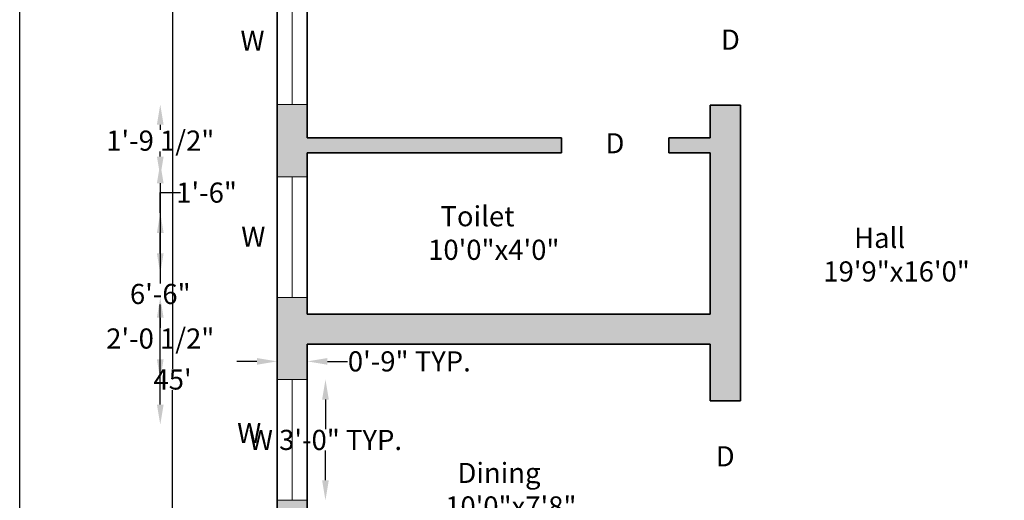
# Model space of a CAD drawing. Units: inches. Extents: x 1054 to 1577, y 4847 to 5610.
# Tile 3 of 5: x 1054 to 1347, y 5221 to 5365. Entities that reach past the tile are written whole.
import ezdxf

# ---------------------------------------------------------------- set-up
doc = ezdxf.new("R2010")
doc.units = ezdxf.units.IN
doc.header["$MEASUREMENT"] = 0
for name, color, linetype, lineweight in [('A-ANNO-DIMS', 2, 'Continuous', 18), ('A-ANNO-TEXT', 7, 'Continuous', 18), ('A-ANNO-TTLB', 7, 'Continuous', 25), ('A-AREA-IDEN', 7, 'Continuous', 18), ('A-GLAZ', 4, 'Continuous', 18), ('A-WALL', 7, 'Continuous', 35)]:
    doc.layers.add(name, color=color, linetype=linetype, lineweight=lineweight)
doc.layers.add('A-WALL-PATT', color=240, linetype='Continuous', lineweight=13, true_color=0xed1f24)
doc.styles.get("Standard").update_dxf_attribs({"font": 'arial.ttf'})
doc.dimstyles.get("Standard").update_dxf_attribs({"dimtxt": 6, "dimasz": 6, "dimexe": 0.18, "dimexo": 0.0625, "dimgap": 0.09, "dimtad": 0, "dimtih": 1, "dimtoh": 1, "dimdec": 1, "dimzin": 0, "dimdsep": 46, "dimlunit": 3, "dimtxsty": 'Standard', "dimcen": 0.09, "dimse1": 1, "dimse2": 1, "dimadec": 0, "dimazin": 0, "dimtfac": 1, "dimtdec": 1, "dimtofl": 0, "dimtmove": 0, "dimatfit": 3, "dimfxl": 1, "dimtolj": 1, "dimtzin": 0, "dimarcsym": 0})

# ---------------------------------------------------------------- blocks, each defined once
blk = doc.blocks.new('*D5')
at = {"layer": 'A-ANNO-DIMS', "color": 0, "lineweight": -2, "transparency": 16777216}
for p, q in [((1099.63, 5521.48), (1099.63, 5260.62)), ((1099.63, 4993.48), (1099.63, 5254.34))]:
    blk.add_line(p, q, dxfattribs=at)
at = {"layer": 'A-ANNO-DIMS', "color": 0, "transparency": 16777216}
for points in [[(1098.63, 5521.48), (1100.63, 5521.48), (1099.63, 5527.48)], [(1098.63, 4993.48), (1100.63, 4993.48), (1099.63, 4987.48)]]:
    blk.add_solid(points, dxfattribs=at)
at = {"layer": 'Defpoints', "color": 0, "transparency": 16777216}
for p in [(1130.77, 5527.48), (1099.63, 4987.48), (1130.77, 4987.48)]:
    blk.add_point(p, dxfattribs=at)
at = {"layer": 'A-ANNO-DIMS', "color": 0, "transparency": 16777216, "insert": (1099.63, 5257.48), "char_height": 6, "attachment_point": 5}
blk.add_mtext("\\A1;45'", dxfattribs=at)
blk = doc.blocks.new('WINDOW-36IN')
for p, q in [((0, 9), (0, 0)), ((36, 9), (0, 9)), ((36, 0), (36, 9)), ((36, 4.5), (0, 4.5)), ((0, 0), (36, 0))]:
    blk.add_line(p, q)
blk = doc.blocks.new('*D10')
at = {"layer": 'A-ANNO-DIMS', "color": 0, "lineweight": -2, "transparency": 16777216}
for p, q in [((1145.17, 5251.48), (1145.17, 5242.64)), ((1145.17, 5227.48), (1145.17, 5236.33))]:
    blk.add_line(p, q, dxfattribs=at)
at = {"layer": 'A-ANNO-DIMS', "color": 0, "transparency": 16777216}
for points in [[(1144.17, 5251.48), (1146.17, 5251.48), (1145.17, 5257.48)], [(1144.17, 5227.48), (1146.17, 5227.48), (1145.17, 5221.48)]]:
    blk.add_solid(points, dxfattribs=at)
at = {"layer": 'Defpoints', "color": 0, "transparency": 16777216}
for p in [(1139.77, 5257.48), (1139.77, 5221.48), (1145.17, 5221.48)]:
    blk.add_point(p, dxfattribs=at)
at = {"layer": 'A-ANNO-DIMS', "color": 0, "transparency": 16777216, "insert": (1145.17, 5239.48), "char_height": 6, "attachment_point": 5}
blk.add_mtext('\\A1;W 3\'-0" TYP.', dxfattribs=at)
blk = doc.blocks.new('*D11')
at = {"layer": 'A-ANNO-DIMS', "color": 0, "lineweight": -2, "transparency": 16777216}
for p, q in [((1124.77, 5262.88), (1118.77, 5262.88)), ((1145.77, 5262.88), (1151.77, 5262.88))]:
    blk.add_line(p, q, dxfattribs=at)
at = {"layer": 'A-ANNO-DIMS', "color": 0, "transparency": 16777216}
for points in [[(1124.77, 5263.88), (1124.77, 5261.88), (1130.77, 5262.88)], [(1145.77, 5263.88), (1145.77, 5261.88), (1139.77, 5262.88)]]:
    blk.add_solid(points, dxfattribs=at)
at = {"layer": 'Defpoints', "color": 0, "transparency": 16777216}
for p in [(1139.77, 5262.88), (1130.77, 5257.48), (1139.77, 5257.48)]:
    blk.add_point(p, dxfattribs=at)
at = {"layer": 'A-ANNO-DIMS', "color": 0, "transparency": 16777216, "insert": (1170.15, 5262.88), "char_height": 6, "attachment_point": 5}
blk.add_mtext('\\A1;0\'-9" TYP.', dxfattribs=at)
blk = doc.blocks.new('*D25')
at = {"layer": 'A-ANNO-DIMS', "color": 0, "lineweight": -2, "transparency": 16777216}
for p, q in [((1348.59, 4855.83), (1352.52, 4855.83)), ((1372.59, 4855.83), (1368.65, 4855.83))]:
    blk.add_line(p, q, dxfattribs=at)
at = {"layer": 'A-ANNO-DIMS', "color": 0, "transparency": 16777216}
for points in [[(1348.59, 4856.83), (1348.59, 4854.83), (1342.59, 4855.83)], [(1372.59, 4856.83), (1372.59, 4854.83), (1378.59, 4855.83)]]:
    blk.add_solid(points, dxfattribs=at)
at = {"layer": 'Defpoints', "color": 0, "transparency": 16777216}
for p in [(1342.59, 5389.48), (1378.59, 5389.48), (1378.59, 4855.83)]:
    blk.add_point(p, dxfattribs=at)
at = {"layer": 'A-ANNO-DIMS', "color": 0, "transparency": 16777216, "insert": (1360.59, 4855.83), "char_height": 6, "attachment_point": 5}
blk.add_mtext('\\A1;3\'-0"', dxfattribs=at)
blk = doc.blocks.new('*D26')
at = {"layer": 'A-ANNO-DIMS', "color": 0, "lineweight": -2, "transparency": 16777216}
for p, q in [((1221.44, 4855.83), (1223.32, 4855.83)), ((1241.44, 4855.83), (1239.56, 4855.83))]:
    blk.add_line(p, q, dxfattribs=at)
at = {"layer": 'A-ANNO-DIMS', "color": 0, "transparency": 16777216}
for points in [[(1221.44, 4856.83), (1221.44, 4854.83), (1215.44, 4855.83)], [(1241.44, 4856.83), (1241.44, 4854.83), (1247.44, 4855.83)]]:
    blk.add_solid(points, dxfattribs=at)
at = {"layer": 'Defpoints', "color": 0, "transparency": 16777216}
for p in [(1215.44, 5324.98), (1247.44, 5324.98), (1247.44, 4855.83)]:
    blk.add_point(p, dxfattribs=at)
at = {"layer": 'A-ANNO-DIMS', "color": 0, "transparency": 16777216, "insert": (1231.44, 4855.83), "char_height": 6, "attachment_point": 5}
blk.add_mtext('\\A1;2\'-8"', dxfattribs=at)
blk = doc.blocks.new('*D33')
at = {"layer": 'A-ANNO-DIMS', "color": 0, "lineweight": -2, "transparency": 16777216}
for p, q in [((1095.97, 5275.9), (1095.97, 5272.88)), ((1095.97, 5263.48), (1095.97, 5266.5))]:
    blk.add_line(p, q, dxfattribs=at)
at = {"layer": 'A-ANNO-DIMS', "color": 0, "transparency": 16777216}
for points in [[(1094.97, 5275.9), (1096.97, 5275.9), (1095.97, 5281.9)], [(1094.97, 5263.48), (1096.97, 5263.48), (1095.97, 5257.48)]]:
    blk.add_solid(points, dxfattribs=at)
at = {"layer": 'Defpoints', "color": 0, "transparency": 16777216}
for p in [(1095.97, 5281.9), (1130.77, 5281.9), (1130.77, 5257.48)]:
    blk.add_point(p, dxfattribs=at)
at = {"layer": 'A-ANNO-DIMS', "color": 0, "transparency": 16777216, "insert": (1095.97, 5269.69), "char_height": 6, "attachment_point": 5}
blk.add_mtext('\\A1;2\'-0 1/2"', dxfattribs=at)
blk = doc.blocks.new('*D34')
at = {"layer": 'A-ANNO-DIMS', "color": 0, "lineweight": -2, "transparency": 16777216}
for p, q in [((1095.97, 5333.41), (1095.97, 5331.85)), ((1095.97, 5323.9), (1095.97, 5325.46))]:
    blk.add_line(p, q, dxfattribs=at)
at = {"layer": 'A-ANNO-DIMS', "color": 0, "transparency": 16777216}
for points in [[(1094.97, 5333.41), (1096.97, 5333.41), (1095.97, 5339.41)], [(1094.97, 5323.9), (1096.97, 5323.9), (1095.97, 5317.9)]]:
    blk.add_solid(points, dxfattribs=at)
at = {"layer": 'Defpoints', "color": 0, "transparency": 16777216}
for p in [(1095.97, 5339.41), (1130.77, 5339.41), (1130.77, 5317.9)]:
    blk.add_point(p, dxfattribs=at)
at = {"layer": 'A-ANNO-DIMS', "color": 0, "transparency": 16777216, "insert": (1095.97, 5328.66), "char_height": 6, "attachment_point": 5}
blk.add_mtext('\\A1;1\'-9 1/2"', dxfattribs=at)
blk = doc.blocks.new('*D39')
at = {"layer": 'A-ANNO-DIMS', "color": 0, "lineweight": -2, "transparency": 16777216}
for p, q in [((1181.77, 5562.28), (1207.69, 5562.28)), ((1249.77, 5562.28), (1223.86, 5562.28))]:
    blk.add_line(p, q, dxfattribs=at)
at = {"layer": 'A-ANNO-DIMS', "color": 0, "transparency": 16777216}
for points in [[(1181.77, 5563.28), (1181.77, 5561.28), (1175.77, 5562.28)], [(1249.77, 5563.28), (1249.77, 5561.28), (1255.77, 5562.28)]]:
    blk.add_solid(points, dxfattribs=at)
at = {"layer": 'Defpoints', "color": 0, "transparency": 16777216}
for p in [(1255.77, 5562.28), (1175.77, 4996.48), (1255.77, 4996.48)]:
    blk.add_point(p, dxfattribs=at)
at = {"layer": 'A-ANNO-DIMS', "color": 0, "transparency": 16777216, "insert": (1215.77, 5562.28), "char_height": 6, "attachment_point": 5}
blk.add_mtext('\\A1;6\'-8"', dxfattribs=at)
blk = doc.blocks.new('*D40')
at = {"layer": 'A-ANNO-DIMS', "color": 0, "lineweight": -2, "transparency": 16777216}
for p, q in [((1145.77, 5562.28), (1149.71, 5562.28)), ((1169.77, 5562.28), (1165.84, 5562.28))]:
    blk.add_line(p, q, dxfattribs=at)
at = {"layer": 'A-ANNO-DIMS', "color": 0, "transparency": 16777216}
for points in [[(1145.77, 5563.28), (1145.77, 5561.28), (1139.77, 5562.28)], [(1169.77, 5563.28), (1169.77, 5561.28), (1175.77, 5562.28)]]:
    blk.add_solid(points, dxfattribs=at)
at = {"layer": 'Defpoints', "color": 0, "transparency": 16777216}
for p in [(1175.77, 5562.28), (1139.77, 4996.48), (1175.77, 4996.48)]:
    blk.add_point(p, dxfattribs=at)
at = {"layer": 'A-ANNO-DIMS', "color": 0, "transparency": 16777216, "insert": (1157.77, 5562.28), "char_height": 6, "attachment_point": 5}
blk.add_mtext('\\A1;3\'-0"', dxfattribs=at)
blk = doc.blocks.new('*D41')
at = {"layer": 'A-ANNO-DIMS', "color": 0, "lineweight": -2, "transparency": 16777216}
for p, q in [((1239.77, 5562.28), (1233.77, 5562.28)), ((1261.77, 5562.28), (1267.77, 5562.28))]:
    blk.add_line(p, q, dxfattribs=at)
at = {"layer": 'A-ANNO-DIMS', "color": 0, "transparency": 16777216}
for points in [[(1239.77, 5563.28), (1239.77, 5561.28), (1245.77, 5562.28)], [(1261.77, 5563.28), (1261.77, 5561.28), (1255.77, 5562.28)]]:
    blk.add_solid(points, dxfattribs=at)
at = {"layer": 'Defpoints', "color": 0, "transparency": 16777216}
for p in [(1255.77, 5562.28), (1245.77, 4996.48), (1255.77, 4996.48)]:
    blk.add_point(p, dxfattribs=at)
at = {"layer": 'A-ANNO-DIMS', "color": 0, "transparency": 16777216, "insert": (1278.17, 5562.28), "char_height": 6, "attachment_point": 5}
blk.add_mtext('\\A1;0\'-10"', dxfattribs=at)
blk = doc.blocks.new('*D46')
at = {"layer": 'A-ANNO-DIMS', "color": 0, "lineweight": -2, "transparency": 16777216}
for p, q in [((1145.77, 4855.83), (1162.54, 4855.83)), ((1209.44, 4855.83), (1192.68, 4855.83))]:
    blk.add_line(p, q, dxfattribs=at)
at = {"layer": 'A-ANNO-DIMS', "color": 0, "transparency": 16777216}
for points in [[(1145.77, 4856.83), (1145.77, 4854.83), (1139.77, 4855.83)], [(1209.44, 4856.83), (1209.44, 4854.83), (1215.44, 4855.83)]]:
    blk.add_solid(points, dxfattribs=at)
at = {"layer": 'Defpoints', "color": 0, "transparency": 16777216}
for p in [(1139.77, 5324.98), (1215.44, 5324.98), (1215.44, 4855.83)]:
    blk.add_point(p, dxfattribs=at)
at = {"layer": 'A-ANNO-DIMS', "color": 0, "transparency": 16777216, "insert": (1177.61, 4855.83), "char_height": 6, "attachment_point": 5}
blk.add_mtext('\\A1;6\'-3 1/2"', dxfattribs=at)
blk = doc.blocks.new('*D47')
at = {"layer": 'A-ANNO-DIMS', "color": 0, "lineweight": -2, "transparency": 16777216}
for p, q in [((1242.78, 5562.28), (1236.78, 5562.28)), ((1265.77, 5562.28), (1271.77, 5562.28))]:
    blk.add_line(p, q, dxfattribs=at)
at = {"layer": 'A-ANNO-DIMS', "color": 0, "transparency": 16777216}
for points in [[(1242.78, 5563.28), (1242.78, 5561.28), (1248.78, 5562.28)], [(1265.77, 5563.28), (1265.77, 5561.28), (1259.77, 5562.28)]]:
    blk.add_solid(points, dxfattribs=at)
at = {"layer": 'Defpoints', "color": 0, "transparency": 16777216}
for p in [(1259.77, 5562.28), (1248.78, 5175.98), (1259.77, 5175.98)]:
    blk.add_point(p, dxfattribs=at)
at = {"layer": 'A-ANNO-DIMS', "color": 0, "transparency": 16777216, "insert": (1282.17, 5562.28), "char_height": 6, "attachment_point": 5}
blk.add_mtext('\\A1;0\'-11"', dxfattribs=at)
blk = doc.blocks.new('*D49')
at = {"layer": 'A-ANNO-DIMS', "color": 0, "lineweight": -2, "transparency": 16777216}
for p, q in [((1095.97, 5307.18), (1095.97, 5313.18)), ((1095.97, 5313.18), (1101.97, 5313.18)), ((1095.97, 5295.07), (1095.97, 5301.18))]:
    blk.add_line(p, q, dxfattribs=at)
at = {"layer": 'A-ANNO-DIMS', "color": 0, "transparency": 16777216}
for points in [[(1094.97, 5301.18), (1096.97, 5301.18), (1095.97, 5307.18)], [(1094.97, 5295.07), (1096.97, 5295.07), (1095.97, 5289.07)]]:
    blk.add_solid(points, dxfattribs=at)
at = {"layer": 'Defpoints', "color": 0, "transparency": 16777216}
for p in [(1095.97, 5307.18), (1393.95, 5307.18), (1393.95, 5289.07)]:
    blk.add_point(p, dxfattribs=at)
at = {"layer": 'A-ANNO-DIMS', "color": 0, "transparency": 16777216, "insert": (1109.76, 5313.18), "char_height": 6, "attachment_point": 5}
blk.add_mtext('\\A1;1\'-6"', dxfattribs=at)
blk = doc.blocks.new('*D51')
at = {"layer": 'A-ANNO-DIMS', "color": 0, "lineweight": -2, "transparency": 16777216}
for p, q in [((1095.97, 5315.94), (1095.97, 5286.13)), ((1095.97, 5250.01), (1095.97, 5279.82))]:
    blk.add_line(p, q, dxfattribs=at)
at = {"layer": 'A-ANNO-DIMS', "color": 0, "transparency": 16777216}
for points in [[(1094.97, 5315.94), (1096.97, 5315.94), (1095.97, 5321.94)], [(1094.97, 5250.01), (1096.97, 5250.01), (1095.97, 5244.01)]]:
    blk.add_solid(points, dxfattribs=at)
at = {"layer": 'Defpoints', "color": 0, "transparency": 16777216}
for p in [(1095.97, 5321.94), (1356.88, 5321.94), (1385.65, 5244.01)]:
    blk.add_point(p, dxfattribs=at)
at = {"layer": 'A-ANNO-DIMS', "color": 0, "transparency": 16777216, "insert": (1095.97, 5282.97), "char_height": 6, "attachment_point": 5}
blk.add_mtext('\\A1;6\'-6"', dxfattribs=at)
blk = doc.blocks.new('*D53')
at = {"layer": 'A-ANNO-DIMS', "color": 0, "lineweight": -2, "transparency": 16777216}
for p, q in [((1145.77, 5562.28), (1159.51, 5562.28)), ((1165.51, 5562.28), (1171.51, 5562.28))]:
    blk.add_line(p, q, dxfattribs=at)
at = {"layer": 'A-ANNO-DIMS', "color": 0, "transparency": 16777216}
for points in [[(1145.77, 5563.28), (1145.77, 5561.28), (1139.77, 5562.28)], [(1159.51, 5563.28), (1159.51, 5561.28), (1165.51, 5562.28)]]:
    blk.add_solid(points, dxfattribs=at)
at = {"layer": 'Defpoints', "color": 0, "transparency": 16777216}
for p in [(1165.51, 5562.28), (1165.51, 5077.04), (1139.77, 5075.48)]:
    blk.add_point(p, dxfattribs=at)
at = {"layer": 'A-ANNO-DIMS', "color": 0, "transparency": 16777216, "insert": (1186.62, 5562.28), "char_height": 6, "attachment_point": 5}
blk.add_mtext('\\A1;2\'-1 1/2"', dxfattribs=at)
blk = doc.blocks.new('*D54')
at = {"layer": 'A-ANNO-DIMS', "color": 0, "lineweight": -2, "transparency": 16777216}
for p, q in [((1245.84, 5562.28), (1239.84, 5562.28)), ((1265.77, 5562.28), (1271.77, 5562.28))]:
    blk.add_line(p, q, dxfattribs=at)
at = {"layer": 'A-ANNO-DIMS', "color": 0, "transparency": 16777216}
for points in [[(1245.84, 5563.28), (1245.84, 5561.28), (1251.84, 5562.28)], [(1265.77, 5563.28), (1265.77, 5561.28), (1259.77, 5562.28)]]:
    blk.add_solid(points, dxfattribs=at)
at = {"layer": 'Defpoints', "color": 0, "transparency": 16777216}
for p in [(1259.77, 5562.28), (1251.84, 5080.96), (1259.77, 5075.48)]:
    blk.add_point(p, dxfattribs=at)
at = {"layer": 'A-ANNO-DIMS', "color": 0, "transparency": 16777216, "insert": (1279.84, 5562.28), "char_height": 6, "attachment_point": 5}
blk.add_mtext('\\A1;0\'-8"', dxfattribs=at)

msp = doc.modelspace()

# ---------------------------------------------------------------- hatches: boundary and pattern name
at = {"layer": 'A-WALL-PATT'}
h = msp.add_hatch(color=256, dxfattribs=at)
h.dxf.hatch_style = 1
h.paths.add_polyline_path([(1213.08, 5527.48), (1130.77, 5527.48), (1130.77, 5375.41), (1139.77, 5375.41), (1139.77, 5518.48), (1213.08, 5518.48)])
h.paths.add_polyline_path([(1470.27, 5527.48), (1383.75, 5527.48), (1383.75, 5518.48), (1457.77, 5518.48), (1457.77, 5446.33), (1462.27, 5446.33), (1462.27, 5518.48), (1470.27, 5518.48)], flags=17)
h.paths.add_polyline_path([(1515.27, 5527.48), (1506.27, 5527.48), (1506.27, 5518.48), (1506.27, 5398.48), (1462.27, 5398.48), (1462.27, 5414.33), (1457.77, 5414.33), (1457.77, 5398.48), (1378.59, 5398.48), (1378.59, 5389.48), (1506.27, 5389.48), (1506.27, 5365.03), (1515.27, 5365.03)])
h.paths.add_polyline_path([(1515.27, 5329.03), (1506.27, 5329.03), (1506.27, 5255.01), (1515.27, 5255.01)])
h.paths.add_polyline_path([(1515.27, 5219.01), (1506.27, 5219.01), (1506.27, 5197.48), (1392.52, 5197.48), (1392.52, 5188.48), (1515.27, 5188.48)])
h.paths.add_polyline_path([(1344.52, 5197.48), (1268.77, 5197.48), (1268.77, 5215.14), (1259.77, 5215.14), (1259.77, 5175.98), (1248.78, 5175.98), (1248.78, 5171.48), (1259.77, 5171.48), (1259.77, 5075.48), (1139.77, 5075.48), (1139.77, 5124.09), (1130.77, 5124.09), (1130.77, 4987.48), (1268.77, 4987.48), (1268.77, 4996.48), (1139.77, 4996.48), (1139.77, 5066.48), (1175.77, 5066.48), (1268.77, 5066.48), (1268.77, 5188.48), (1344.52, 5188.48)])
h.paths.add_polyline_path([(1216.78, 5175.98), (1139.77, 5175.98), (1139.77, 5221.48), (1130.77, 5221.48), (1130.77, 5160.09), (1139.77, 5160.09), (1139.77, 5171.48), (1216.78, 5171.48)])
h.paths.add_polyline_path([(1268.77, 5339.26), (1259.77, 5339.26), (1259.77, 5329.48), (1247.44, 5329.48), (1247.44, 5324.98), (1259.77, 5324.98), (1259.77, 5276.98), (1139.77, 5276.98), (1139.77, 5281.9), (1130.77, 5281.9), (1130.77, 5257.48), (1139.77, 5257.48), (1139.77, 5267.98), (1259.77, 5267.98), (1259.77, 5251.14), (1268.77, 5251.14)])
h.paths.add_polyline_path([(1139.77, 5339.41), (1130.77, 5339.41), (1130.77, 5317.9), (1139.77, 5317.9), (1139.77, 5324.98), (1215.44, 5324.98), (1215.44, 5329.48), (1139.77, 5329.48)])
h.paths.add_polyline_path([(1280.67, 5389.48), (1280.67, 5391.1), (1320.18, 5391.1), (1320.18, 5389.48), (1342.59, 5389.48), (1342.59, 5398.48), (1268.77, 5398.48), (1268.77, 5518.48), (1347.75, 5518.48), (1347.75, 5527.48), (1249.08, 5527.48), (1249.08, 5518.48), (1259.77, 5518.48), (1259.77, 5375.26), (1268.77, 5375.26), (1268.77, 5389.48)])

# ---------------------------------------------------------------- linework, layer by layer
at = {"layer": 'A-ANNO-TTLB'}
msp.add_lwpolyline([(1054.1, 5610.1), (1577.31, 5610.1), (1577.31, 4927.21), (1054.1, 4927.21)], close=True, dxfattribs=at)
at = {"layer": 'A-WALL'}
for p, q in [((1130.77, 5527.48), (1130.77, 4987.48)), ((1139.77, 5518.48), (1139.77, 5329.48)), ((1268.77, 5339.26), (1259.77, 5339.26)), ((1259.77, 5339.26), (1259.77, 5329.48)), ((1268.77, 5339.26), (1268.77, 5251.14)), ((1139.77, 5329.48), (1215.44, 5329.48)), ((1215.44, 5324.98), (1215.44, 5329.48)), ((1247.44, 5329.48), (1247.44, 5324.98)), ((1247.44, 5329.48), (1259.77, 5329.48)), ((1139.77, 5324.98), (1215.44, 5324.98)), ((1139.77, 5324.98), (1139.77, 5276.98)), ((1247.44, 5324.98), (1259.77, 5324.98)), ((1259.77, 5324.98), (1259.77, 5276.98)), ((1139.77, 5276.98), (1259.77, 5276.98)), ((1139.77, 5267.98), (1259.77, 5267.98)), ((1139.77, 5267.98), (1139.77, 5175.98)), ((1259.77, 5267.98), (1259.77, 5251.14)), ((1259.77, 5251.14), (1268.77, 5251.14))]:
    msp.add_line(p, q, dxfattribs=at)

# ---------------------------------------------------------------- block references
at = {"layer": 'A-GLAZ'}
for p, rotation in [((1139.77, 5339.41), 89.99999999999471), ((1130.77, 5317.9), 269.9999999999954), ((1130.77, 5257.48), 269.9999999999961)]:
    msp.add_blockref('WINDOW-36IN', p, dxfattribs=dict(at, rotation=rotation))

# ---------------------------------------------------------------- texts
at = {"layer": 'A-ANNO-TEXT', "char_height": 6, "attachment_point": 1}
for s, width, insert in [('W', 11.4277, (1119.84, 5361.44)), ('D', 9.0631, (1262.97, 5361.76)), ('D', 9.0631, (1228.59, 5330.88)), ('W', 11.4277, (1120.09, 5303.02)), ('W', 11.4277, (1118.86, 5244.56)), ('D', 9.0631, (1261.42, 5237.6))]:
    msp.add_mtext_dynamic_manual_height_columns(s, width=width, gutter_width=30, heights=[0], dxfattribs=dict(at, insert=insert))
at = {"layer": 'A-AREA-IDEN', "char_height": 6, "attachment_point": 1}
for s, width, insert in [('  Toilet\\P10\'0"x4\'0"', 44.2165, (1175.76, 5309.13)), ('     Hall\\P19\'9"x16\'0"', 45.2362, (1293.46, 5302.68)), ('  Dining\\P10\'0"x7\'8"', 62.8209, (1180.83, 5232.65))]:
    msp.add_mtext_dynamic_manual_height_columns(s, width=width, gutter_width=30, heights=[0], dxfattribs=dict(at, insert=insert))

# ---------------------------------------------------------------- dimensions: what is measured, and where the dimension line sits
at = {"layer": 'A-ANNO-DIMS'}
for base, p1, p2, picture, middle in [((1165.51, 5562.28), (1139.77, 5075.48), (1165.51, 5077.04), '*D53', (1186.62, 5562.28)), ((1175.77, 5562.28), (1139.77, 4996.48), (1175.77, 4996.48), '*D40', (1157.77, 5562.28)), ((1255.77, 5562.28), (1175.77, 4996.48), (1255.77, 4996.48), '*D39', (1215.77, 5562.28)), ((1255.77, 5562.28), (1245.77, 4996.48), (1255.77, 4996.48), '*D41', (1278.17, 5562.28)), ((1259.77, 5562.28), (1248.78, 5175.98), (1259.77, 5175.98), '*D47', (1282.17, 5562.28)), ((1259.77, 5562.28), (1251.84, 5080.96), (1259.77, 5075.48), '*D54', (1279.84, 5562.28)), ((1378.59, 4855.83), (1342.59, 5389.48), (1378.59, 5389.48), '*D25', (1360.59, 4855.83)), ((1215.44, 4855.83), (1139.77, 5324.98), (1215.44, 5324.98), '*D46', (1177.61, 4855.83)), ((1247.44, 4855.83), (1215.44, 5324.98), (1247.44, 5324.98), '*D26', (1231.44, 4855.83))]:
    dim = msp.add_linear_dim(base=base, p1=p1, p2=p2, dimstyle='Standard', override={"dimdec": 1, "dimlfac": 1, "dimrnd": 0, "dimzin": 1, "dimdsep": 46, "dimlunit": 4, "dimfrac": 2}, dxfattribs=at)
    dim.commit()
    dim.dimension.update_dxf_attribs({"geometry": picture, "text_midpoint": middle})
for base, p1, p2, override, picture, middle in [((1099.63, 4987.48), (1130.77, 5527.48), (1130.77, 4987.48), {"dimclrd": 0, "dimclre": 0, "dimclrt": 0}, '*D5', (1099.63, 5257.48)), ((1095.97, 5339.41), (1130.77, 5317.9), (1130.77, 5339.41), {"dimdec": 1, "dimlfac": 1, "dimrnd": 0, "dimzin": 1, "dimdsep": 46, "dimlunit": 4, "dimfrac": 2}, '*D34', (1095.97, 5328.66)), ((1095.97, 5321.94), (1385.65, 5244.01), (1356.88, 5321.94), {"dimdec": 1, "dimlfac": 1, "dimrnd": 0, "dimzin": 1, "dimdsep": 46, "dimlunit": 4, "dimfrac": 2}, '*D51', (1095.97, 5282.97)), ((1095.97, 5307.18), (1393.95, 5289.07), (1393.95, 5307.18), {"dimdec": 1, "dimlfac": 1, "dimrnd": 0, "dimzin": 1, "dimdsep": 46, "dimlunit": 4, "dimfrac": 2}, '*D49', (1109.76, 5313.18)), ((1095.97, 5281.9), (1130.77, 5257.48), (1130.77, 5281.9), {"dimdec": 1, "dimlfac": 1, "dimrnd": 0, "dimzin": 1, "dimdsep": 46, "dimlunit": 4, "dimfrac": 2}, '*D33', (1095.97, 5269.69))]:
    dim = msp.add_linear_dim(base=base, p1=p1, p2=p2, angle=90, dimstyle='Standard', override=override, dxfattribs=at)
    dim.commit()
    dim.dimension.update_dxf_attribs({"geometry": picture, "text_midpoint": middle})
dim = msp.add_linear_dim(base=(1139.77, 5262.88), p1=(1130.77, 5257.48), p2=(1139.77, 5257.48), text='<> TYP.', dimstyle='Standard', override={"dimdec": 1, "dimlfac": 1, "dimrnd": 0, "dimzin": 1, "dimdsep": 46, "dimlunit": 4, "dimfrac": 2}, dxfattribs=at)
dim.commit()
dim.dimension.update_dxf_attribs({"geometry": '*D11', "text_midpoint": (1170.15, 5262.88)})
dim = msp.add_linear_dim(base=(1145.17, 5221.48), p1=(1139.77, 5257.48), p2=(1139.77, 5221.48), angle=270, text='W <> TYP.', dimstyle='Standard', override={"dimdec": 1, "dimlfac": 1, "dimrnd": 0, "dimzin": 1, "dimdsep": 46, "dimlunit": 4, "dimfrac": 2}, dxfattribs=at)
dim.commit()
dim.dimension.update_dxf_attribs({"geometry": '*D10', "text_midpoint": (1145.17, 5239.48)})

doc.saveas('drawing.dxf')
